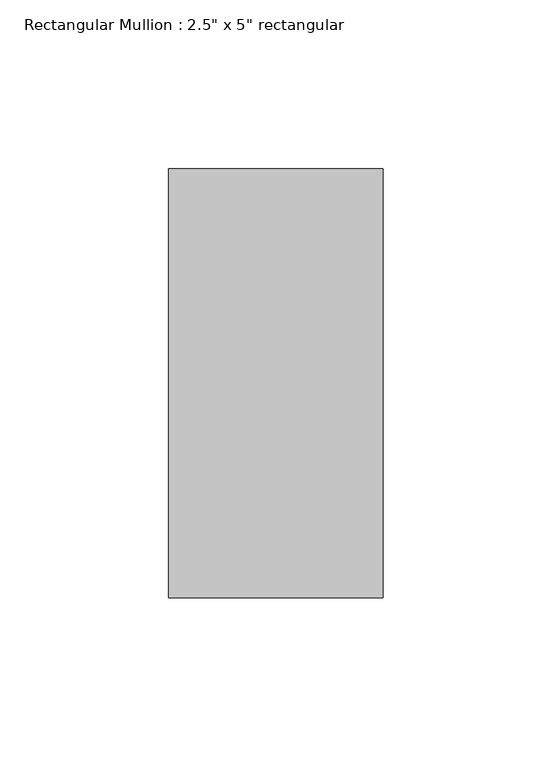
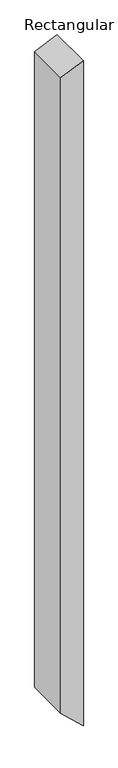
"""IFC4 building model written with IfcOpenShell, lengths in millimetres: member geometry."""

from ifc_helpers import new_model, si_unit, frame, origin, place, context, project, spatial, polyline, outline, extrude, source, transform, mapped, element, save


def member_d36c5697(model_context):
    return source(origin(), model_context, "Body", "SweptSolid", [
        extrude(outline(polyline([(0.0, 0.0), (-27.6105858, -63.5), (-1918.5971803, -63.5), (-1977.8118883, 0.0), (0.0, 0.0)])), frame((0.0, -63.5, 0.0), z_axis=(0.0, 1.0, 0.0), x_axis=(0.0, 0.0, 1.0)), (0.0, 0.0, 1.0), 127.0),
    ])


if __name__ == "__main__":
    model = new_model("IFC4")
    model_context = context("Model", 3, world=origin())
    ifc_project = project(units=[si_unit("LENGTHUNIT", "METRE", prefix="MILLI")], contexts=[model_context])
    site = spatial("IfcSite", under=ifc_project)
    building = spatial("IfcBuilding", under=site)
    placement = place(None, origin())
    member_shape = member_d36c5697(model_context)
    element("IfcMember", 1, ObjectType="Rectangular Mullion : 2.5\" x 5\" rectangular", at=placement, inside=building, context=model_context, shape_type="MappedRepresentation", body=[
        mapped(member_shape, transform((0.0, 0.0, 0.0), x_axis=(1.0, 0.0, 0.0), y_axis=(0.0, 1.0, 0.0), z_axis=(0.0, 0.0, 1.0))),
    ])
    save(model, "model.ifc")

# Revit data of these elements
# Type "Rectangular Mullion : 2.5\" x 5\" rectangular"
#   built-in parameter 1007304 = 0.416667 (stored number, unit not read)
#   built-in parameter 1007301 = 0.104167 (stored number, unit not read)
#   built-in parameter 1007300 = 0.104167 (stored number, unit not read)
# Element 1 (IfcMember, "Rectangular Mullion : 2.5\" x 5\" rectangular")
#   Materials on its faces: "door colour"
# Materials
#   "door colour": class "Generic", colour RGB 120 120 120, transparency 0, Cost = 0
